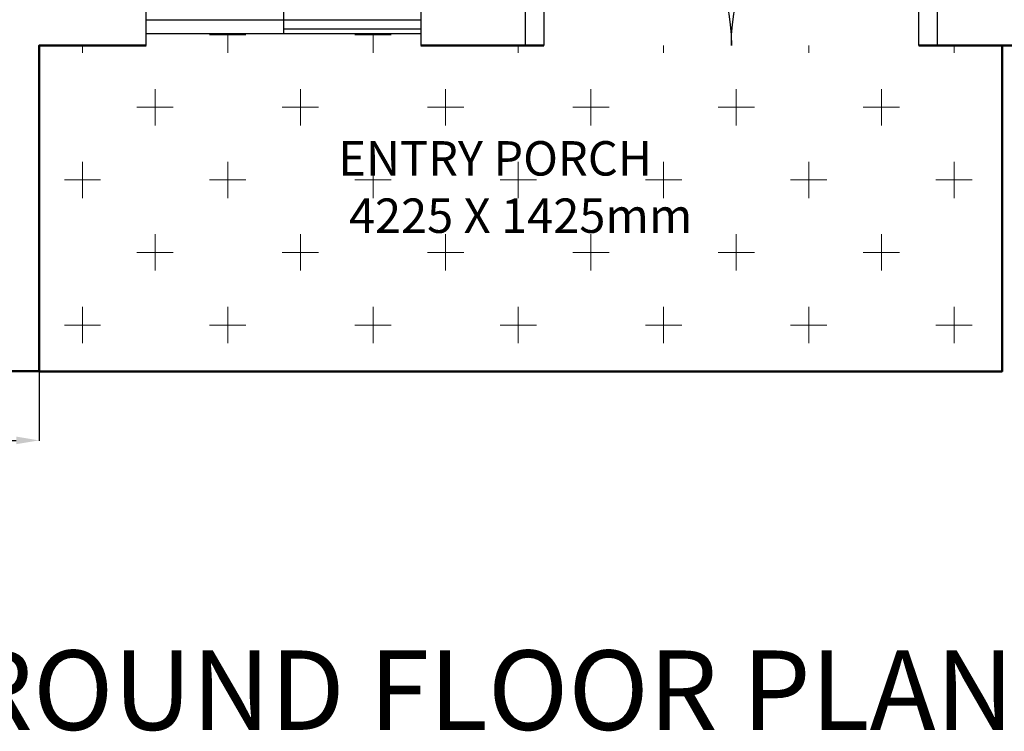
# Model space of a CAD drawing. Units: millimetres. Extents: x -857 to 54106, y -13666 to 13947.
# Tile 3 of 41: x 7333 to 11637, y 2329 to 5442. Entities that reach past the tile are written whole.
import ezdxf

# ---------------------------------------------------------------- set-up
doc = ezdxf.new("R2010")
doc.units = ezdxf.units.MM
for name, color, linetype, lineweight in [('A-ANNO-DIMS', 2, 'Continuous', 18), ('A-ANNO-TEXT', 7, 'Continuous', 25), ('A-AREA-IDEN', 3, 'Continuous', 18), ('A-DOOR', 1, 'Continuous', 25), ('A-FLOR-PATT', 252, 'Continuous', 13), ('A-GLAZ', 4, 'Continuous', 25), ('A-WALL', 7, 'Continuous', 50)]:
    doc.layers.add(name, color=color, linetype=linetype, lineweight=lineweight)
doc.styles.get("Standard").update_dxf_attribs({"font": 'arial.ttf'})
doc.dimstyles.new('ISO-25', dxfattribs={"dimtxt": 2.5, "dimasz": 2.5, "dimexe": 1.25, "dimexo": 0.625, "dimtad": 1, "dimtxsty": 'Standard', "dimcen": 2.5, "dimadec": 0, "dimazin": 0, "dimtfac": 1, "dimtmove": 0, "dimatfit": 3, "dimfxl": 1, "dimarcsym": 0})

# ---------------------------------------------------------------- blocks, each defined once
blk = doc.blocks.new('*D24')
at = {"layer": 'A-ANNO-DIMS', "color": 0, "lineweight": -2, "transparency": 16777216}
for p, q in [((3567.3, 3903.6), (3567.3, 3600.6)), ((7417.3, 3903.2), (7417.3, 3600.6)), ((3667.3, 3601.8), (7317.3, 3601.8))]:
    blk.add_line(p, q, dxfattribs=at)
at = {"layer": 'A-ANNO-DIMS', "color": 0, "transparency": 16777216}
for points in [[(3667.3, 3618.5), (3667.3, 3585.1), (3567.3, 3601.8)], [(7317.3, 3618.5), (7317.3, 3585.1), (7417.3, 3601.8)]]:
    blk.add_solid(points, dxfattribs=at)
at = {"layer": 'Defpoints', "color": 0, "transparency": 16777216}
for p in [(3567.3, 3904.3), (7417.3, 3903.8), (7417.3, 3601.8)]:
    blk.add_point(p, dxfattribs=at)
at = {"layer": 'A-ANNO-DIMS', "color": 0, "transparency": 16777216, "insert": (5492.3, 3653.5), "char_height": 100, "attachment_point": 5}
blk.add_mtext('3850', dxfattribs=at)
blk = doc.blocks.new('WIN-1200')
for p, q in [((9371.3, 11750.2), (10571.3, 11750.2)), ((9371.3, 11731.7), (9971.3, 11731.7)), ((9971.3, 11750.2), (9971.3, 11630.7)), ((9371.3, 11691.7), (10571.3, 11691.7)), ((10571.3, 11630.7), (9371.3, 11630.7)), ((9971.3, 11651.7), (10571.3, 11651.7))]:
    blk.add_line(p, q)
for points in [[(9371.3, 11579.2), (9371.3, 11804.2)], [(10571.3, 11804.2), (10571.3, 11579.2)]]:
    blk.add_lwpolyline(points)

msp = doc.modelspace()

# ---------------------------------------------------------------- hatches: boundary and pattern name
at = {"layer": 'A-FLOR-PATT'}
h = msp.add_hatch(dxfattribs=at)
h.set_pattern_fill('CROSS', color=256, scale=50)
h.set_pattern_definition([(0, (-5489.92, -2561.3), (317.5, 317.5), [158.75, -476.25]), (90, (-5410.54, -2640.7), (-317.5, 317.5), [158.75, -476.25])])
h.paths.add_polyline_path([(11627.12, 5329.231), (11263.585, 5329.231), (9623.585, 5329.231), (9543.585, 5329.231), (9086.254, 5329.231), (9086.254, 5380.706), (7886.254, 5380.706), (7886.254, 5329.231), (7417.28, 5329.231), (7417.28, 3903.799), (11627.12, 3903.799)])

# ---------------------------------------------------------------- linework, layer by layer
at = {"layer": 'A-DOOR'}
msp.add_lwpolyline([(9623.585, 6229.231), (9623.585, 5329.231), (9543.585, 5329.231), (9543.585, 6229.231, -0.41421356), (10443.585, 5329.231, -0.41421356), (11343.585, 6229.231), (11343.585, 5329.231), (11263.585, 5329.231), (11263.585, 6229.231)], format="xyb", dxfattribs=at)
at = {"layer": 'A-WALL'}
msp.add_line((6140.719, 3904.023), (7417.28, 3904.023), dxfattribs=at)
for points in [[(7886.254, 5329.231), (7417.28, 5329.231), (7417.28, 3903.799), (11627.12, 3903.799), (11627.12, 5329.231), (11263.585, 5329.231)], [(7886.254, 5329.231), (7417.28, 5329.231), (7417.28, 3903.799)], [(9623.585, 5329.231), (9086.254, 5329.231)], [(9623.585, 5329.231), (9086.254, 5329.231)], [(12200.793, 5329.231), (11263.585, 5329.231)]]:
    msp.add_lwpolyline(points, dxfattribs=at)

# ---------------------------------------------------------------- block references
at = {"layer": 'A-GLAZ'}
msp.add_blockref('WIN-1200', (-1485.087, -6250), dxfattribs=at)

# ---------------------------------------------------------------- texts
at = {"layer": 'A-ANNO-TEXT', "insert": (6763.058, 2682.963), "char_height": 347.60543, "attachment_point": 1}
msp.add_mtext_dynamic_manual_height_columns('\\pxt0;GROUND FLOOR PLAN', width=5900.0263, gutter_width=43450.679, heights=[5996.136], dxfattribs=at)
at = {"layer": 'A-AREA-IDEN', "insert": (8725.861, 4910.875), "char_height": 150.48461, "attachment_point": 1}
msp.add_mtext_dynamic_manual_height_columns('\\pxt0;ENTRY PORCH\\P 4225 X 1425mm', width=2554.22693, gutter_width=18810.576, heights=[2595.835], dxfattribs=at)

# ---------------------------------------------------------------- dimensions: what is measured, and where the dimension line sits
at = {"layer": 'A-ANNO-DIMS'}
dim = msp.add_linear_dim(base=(7417.28, 3601.816), p1=(3567.28, 3904.258), p2=(7417.28, 3903.799), dimstyle='ISO-25', override={"dimtxt": 100, "dimasz": 100, "dimclrd": 0, "dimclre": 0, "dimclrt": 0}, dxfattribs=at)
dim.commit()
dim.dimension.update_dxf_attribs({"geometry": '*D24', "text_midpoint": (5492.28, 3653.533)})

doc.saveas('drawing.dxf')
